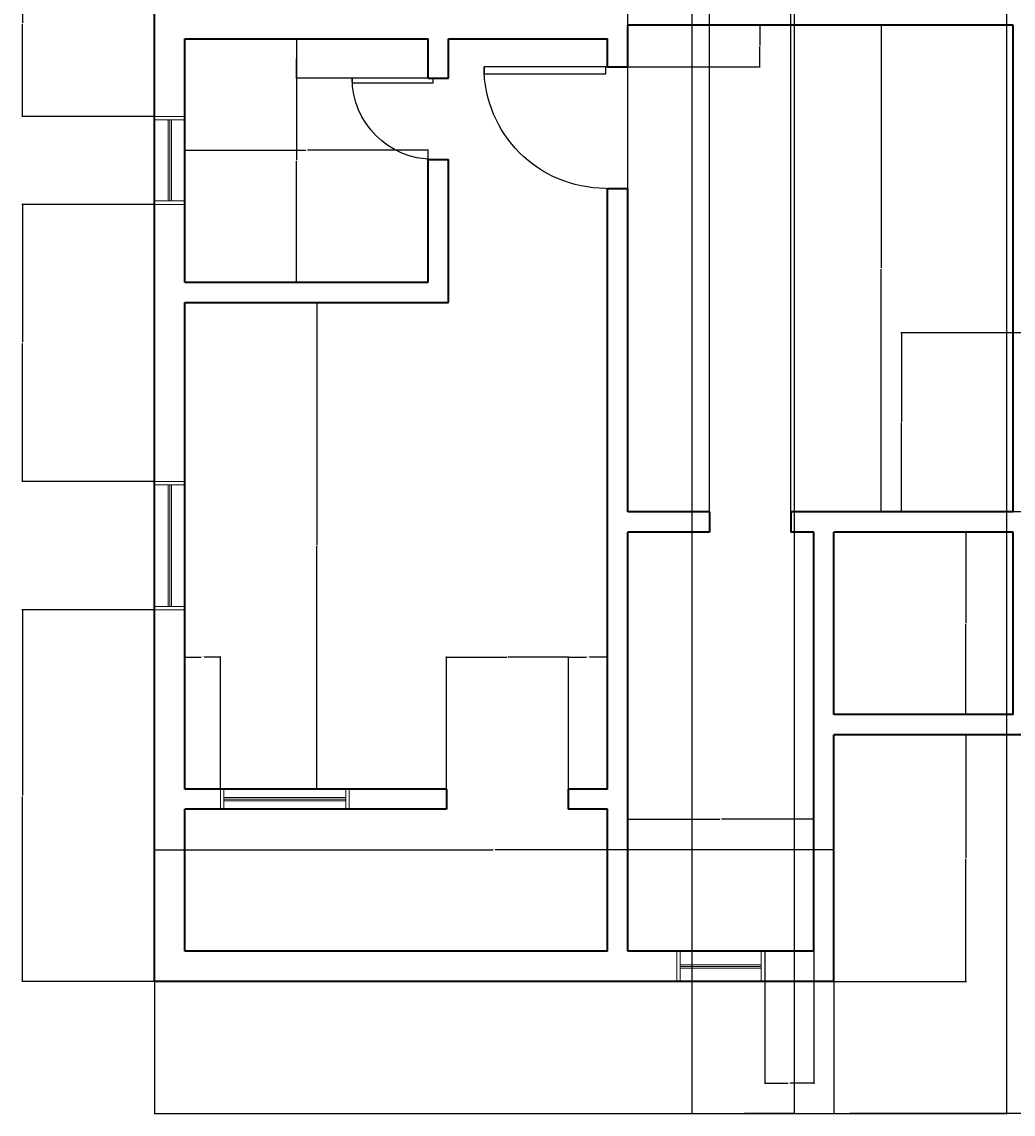
# Model space of a CAD drawing. Units: inches. Extents: x -7288 to -6705, y 7169 to 8028.
# Tile 1 of 5: x -7288 to -6995, y 7169 to 7493. Entities that reach past the tile are written whole.
import ezdxf

# ---------------------------------------------------------------- set-up
doc = ezdxf.new("R2010")
doc.units = ezdxf.units.IN
for name, color, linetype, lineweight in [('A-ANNO-DIMS', 2, 'Continuous', 18), ('A-DOOR', 3, 'Continuous', 25), ('A-GLAZ', 2, 'Continuous', 18), ('A-WALL', 1, 'Continuous', 35)]:
    doc.layers.add(name, color=color, linetype=linetype, lineweight=lineweight)
doc.styles.get("Standard").update_dxf_attribs({"font": 'arial.ttf'})
doc.dimstyles.get("Standard").update_dxf_attribs({"dimtxt": 0.18, "dimasz": 0.18, "dimexe": 0.18, "dimexo": 0.0625, "dimgap": 0.09, "dimtad": 0, "dimtih": 1, "dimtoh": 1, "dimdec": 4, "dimzin": 0, "dimdsep": 46, "dimtxsty": 'Standard', "dimcen": 0.09, "dimadec": 0, "dimazin": 0, "dimtfac": 1, "dimtdec": 4, "dimtofl": 0, "dimtmove": 0, "dimatfit": 3, "dimfxl": 1, "dimtolj": 1, "dimtzin": 0, "dimarcsym": 0})

# ---------------------------------------------------------------- blocks, each defined once
blk = doc.blocks.new('*U8')
for p, q in [((0, 0), (0, -100)), ((750, 0), (750, -100))]:
    blk.add_line(p, q)
blk.add_lwpolyline([(0, 0), (0, 750), (43.75, 750), (43.75, 0)], close=True)
blk.add_arc((0, 0), 750, 0, 90)
blk = doc.blocks.new('WIN-36IN-WALL9')
for p, q in [((0, 38), (9, 38)), ((0, 37), (9, 37)), ((4, 1), (4, 37)), ((4.5, 1), (4.5, 37)), ((5, 1), (5, 37)), ((0, 1), (9, 1)), ((0, 0), (9, 0))]:
    blk.add_line(p, q)
blk = doc.blocks.new('WIN-24IN-WALL9')
for p, q in [((0, 26), (9, 26)), ((0, 25), (9, 25)), ((4, 1), (4, 25)), ((4.5, 1), (4.5, 25)), ((5, 1), (5, 25)), ((0, 1), (9, 1)), ((0, 0), (9, 0))]:
    blk.add_line(p, q)
blk = doc.blocks.new('WIN-36IN-WALL6')
for p, q in [((0, 6), (0, 0)), ((1, 6), (1, 0)), ((1, 3.5), (37, 3.5)), ((37, 6), (37, 0)), ((38, 6), (38, 0)), ((1, 3), (37, 3)), ((1, 2.5), (37, 2.5))]:
    blk.add_line(p, q)
blk = doc.blocks.new('*D93')
at = {"layer": 'A-ANNO-DIMS', "color": 0, "lineweight": -2, "transparency": 16777216}
for p, q in [((-7248.84, 7208.47), (-7248.84, 7169.32)), ((-6744.84, 7208.47), (-6744.84, 7169.32)), ((-7248.66, 7169.5), (-6997.13, 7169.5)), ((-6745.02, 7169.5), (-6996.55, 7169.5))]:
    blk.add_line(p, q, dxfattribs=at)
at = {"layer": 'A-ANNO-DIMS', "color": 0, "transparency": 16777216}
for points in [[(-7248.66, 7169.53), (-7248.66, 7169.47), (-7248.84, 7169.5)], [(-6745.02, 7169.53), (-6745.02, 7169.47), (-6744.84, 7169.5)]]:
    blk.add_solid(points, dxfattribs=at)
at = {"layer": 'Defpoints', "color": 0, "transparency": 16777216}
for p in [(-7248.84, 7208.53), (-6744.84, 7208.53), (-6744.84, 7169.5)]:
    blk.add_point(p, dxfattribs=at)
at = {"layer": 'A-ANNO-DIMS', "color": 0, "transparency": 16777216, "insert": (-6996.84, 7169.5), "char_height": 0.18, "attachment_point": 5}
blk.add_mtext('\\A1;504', dxfattribs=at)
blk = doc.blocks.new('*D100')
at = {"layer": 'A-ANNO-DIMS', "color": 0, "lineweight": -2, "transparency": 16777216}
for p, q in [((-7248.84, 7208.59), (-7248.84, 7247.74)), ((-7248.66, 7247.56), (-7148.61, 7247.56)), ((-7048.02, 7247.56), (-7148.07, 7247.56)), ((-7047.84, 7208.59), (-7047.84, 7247.74))]:
    blk.add_line(p, q, dxfattribs=at)
at = {"layer": 'A-ANNO-DIMS', "color": 0, "transparency": 16777216}
for points in [[(-7248.66, 7247.59), (-7248.66, 7247.53), (-7248.84, 7247.56)], [(-7048.02, 7247.59), (-7048.02, 7247.53), (-7047.84, 7247.56)]]:
    blk.add_solid(points, dxfattribs=at)
at = {"layer": 'Defpoints', "color": 0, "transparency": 16777216}
for p in [(-7047.84, 7247.56), (-7248.84, 7208.53), (-7047.84, 7208.53)]:
    blk.add_point(p, dxfattribs=at)
at = {"layer": 'A-ANNO-DIMS', "color": 0, "transparency": 16777216, "insert": (-7148.34, 7247.56), "char_height": 0.18, "attachment_point": 5}
blk.add_mtext('\\A1;201', dxfattribs=at)
blk = doc.blocks.new('*D101')
at = {"layer": 'A-ANNO-DIMS', "color": 0, "lineweight": -2, "transparency": 16777216}
for p, q in [((-7047.84, 7208.47), (-7047.84, 7169.32)), ((-6945.84, 7208.47), (-6945.84, 7169.32)), ((-7047.66, 7169.5), (-6997.12, 7169.5)), ((-6946.02, 7169.5), (-6996.56, 7169.5))]:
    blk.add_line(p, q, dxfattribs=at)
at = {"layer": 'A-ANNO-DIMS', "color": 0, "transparency": 16777216}
for points in [[(-7047.66, 7169.53), (-7047.66, 7169.47), (-7047.84, 7169.5)], [(-6946.02, 7169.53), (-6946.02, 7169.47), (-6945.84, 7169.5)]]:
    blk.add_solid(points, dxfattribs=at)
at = {"layer": 'Defpoints', "color": 0, "transparency": 16777216}
for p in [(-7047.84, 7208.53), (-6945.84, 7208.53), (-6945.84, 7169.5)]:
    blk.add_point(p, dxfattribs=at)
at = {"layer": 'A-ANNO-DIMS', "color": 0, "transparency": 16777216, "insert": (-6996.84, 7169.5), "char_height": 0.18, "attachment_point": 5}
blk.add_mtext('\\A1;102', dxfattribs=at)
blk = doc.blocks.new('*D102')
at = {"layer": 'A-ANNO-DIMS', "color": 0, "lineweight": -2, "transparency": 16777216}
for p, q in [((-7047.78, 7281.53), (-7008.63, 7281.53)), ((-7008.81, 7281.35), (-7008.81, 7245.21)), ((-7008.81, 7208.71), (-7008.81, 7244.85)), ((-7047.78, 7208.53), (-7008.63, 7208.53))]:
    blk.add_line(p, q, dxfattribs=at)
at = {"layer": 'A-ANNO-DIMS', "color": 0, "transparency": 16777216}
for points in [[(-7008.84, 7281.35), (-7008.78, 7281.35), (-7008.81, 7281.53)], [(-7008.84, 7208.71), (-7008.78, 7208.71), (-7008.81, 7208.53)]]:
    blk.add_solid(points, dxfattribs=at)
at = {"layer": 'Defpoints', "color": 0, "transparency": 16777216}
for p in [(-7047.84, 7281.53), (-7047.84, 7208.53), (-7008.81, 7208.53)]:
    blk.add_point(p, dxfattribs=at)
at = {"layer": 'A-ANNO-DIMS', "color": 0, "transparency": 16777216, "insert": (-7008.81, 7245.03), "char_height": 0.18, "attachment_point": 5}
blk.add_mtext('\\A1;73', dxfattribs=at)
blk = doc.blocks.new('*D103')
at = {"layer": 'A-ANNO-DIMS', "color": 0, "lineweight": -2, "transparency": 16777216}
for p, q in [((-7089.84, 7838.47), (-7089.84, 7169.32)), ((-6996.84, 7838.47), (-6996.84, 7169.32)), ((-7089.66, 7169.5), (-7043.56, 7169.5)), ((-6997.02, 7169.5), (-7043.12, 7169.5))]:
    blk.add_line(p, q, dxfattribs=at)
at = {"layer": 'A-ANNO-DIMS', "color": 0, "transparency": 16777216}
for points in [[(-7089.66, 7169.53), (-7089.66, 7169.47), (-7089.84, 7169.5)], [(-6997.02, 7169.53), (-6997.02, 7169.47), (-6996.84, 7169.5)]]:
    blk.add_solid(points, dxfattribs=at)
at = {"layer": 'Defpoints', "color": 0, "transparency": 16777216}
for p in [(-7089.84, 7838.53), (-6996.84, 7838.53), (-6996.84, 7169.5)]:
    blk.add_point(p, dxfattribs=at)
at = {"layer": 'A-ANNO-DIMS', "color": 0, "transparency": 16777216, "insert": (-7043.34, 7169.5), "char_height": 0.18, "attachment_point": 5}
blk.add_mtext('\\A1;93', dxfattribs=at)
blk = doc.blocks.new('*D119')
at = {"layer": 'A-ANNO-DIMS', "color": 0, "lineweight": -2, "transparency": 16777216}
for p, q in [((-7089.84, 7799.47), (-7089.84, 7169.32)), ((-7059.61, 7799.47), (-7059.61, 7169.32)), ((-7089.66, 7169.5), (-7075.12, 7169.5)), ((-7059.79, 7169.5), (-7074.33, 7169.5))]:
    blk.add_line(p, q, dxfattribs=at)
at = {"layer": 'A-ANNO-DIMS', "color": 0, "transparency": 16777216}
for points in [[(-7089.66, 7169.53), (-7089.66, 7169.47), (-7089.84, 7169.5)], [(-7059.79, 7169.53), (-7059.79, 7169.47), (-7059.61, 7169.5)]]:
    blk.add_solid(points, dxfattribs=at)
at = {"layer": 'Defpoints', "color": 0, "transparency": 16777216}
for p in [(-7089.84, 7799.53), (-7059.61, 7799.53), (-7059.61, 7169.5)]:
    blk.add_point(p, dxfattribs=at)
at = {"layer": 'A-ANNO-DIMS', "color": 0, "transparency": 16777216, "insert": (-7074.72, 7169.5), "char_height": 0.18, "attachment_point": 5}
blk.add_mtext('\\A1;30.23', dxfattribs=at)
blk = doc.blocks.new('*D139')
at = {"layer": 'A-ANNO-DIMS', "color": 0, "lineweight": -2, "transparency": 16777216}
for p, q in [((-6994.9, 7491.53), (-7034.05, 7491.53)), ((-7033.87, 7491.35), (-7033.87, 7419.71)), ((-7033.87, 7347.71), (-7033.87, 7419.35)), ((-6994.9, 7347.53), (-7034.05, 7347.53))]:
    blk.add_line(p, q, dxfattribs=at)
at = {"layer": 'A-ANNO-DIMS', "color": 0, "transparency": 16777216}
for points in [[(-7033.9, 7491.35), (-7033.84, 7491.35), (-7033.87, 7491.53)], [(-7033.9, 7347.71), (-7033.84, 7347.71), (-7033.87, 7347.53)]]:
    blk.add_solid(points, dxfattribs=at)
at = {"layer": 'Defpoints', "color": 0, "transparency": 16777216}
for p in [(-7033.87, 7491.53), (-6994.84, 7491.53), (-6994.84, 7347.53)]:
    blk.add_point(p, dxfattribs=at)
at = {"layer": 'A-ANNO-DIMS', "color": 0, "transparency": 16777216, "insert": (-7033.87, 7419.53), "char_height": 0.18, "attachment_point": 5}
blk.add_mtext('\\A1;144', dxfattribs=at)
blk = doc.blocks.new('*D140')
at = {"layer": 'A-ANNO-DIMS', "color": 0, "lineweight": -2, "transparency": 16777216}
for p, q in [((-7239.84, 7415.59), (-7239.84, 7454.74)), ((-7239.66, 7454.56), (-7204.06, 7454.56)), ((-7168.02, 7454.56), (-7203.62, 7454.56)), ((-7167.84, 7415.59), (-7167.84, 7454.74))]:
    blk.add_line(p, q, dxfattribs=at)
at = {"layer": 'A-ANNO-DIMS', "color": 0, "transparency": 16777216}
for points in [[(-7239.66, 7454.59), (-7239.66, 7454.53), (-7239.84, 7454.56)], [(-7168.02, 7454.59), (-7168.02, 7454.53), (-7167.84, 7454.56)]]:
    blk.add_solid(points, dxfattribs=at)
at = {"layer": 'Defpoints', "color": 0, "transparency": 16777216}
for p in [(-7167.84, 7454.56), (-7239.84, 7415.53), (-7167.84, 7415.53)]:
    blk.add_point(p, dxfattribs=at)
at = {"layer": 'A-ANNO-DIMS', "color": 0, "transparency": 16777216, "insert": (-7203.84, 7454.56), "char_height": 0.18, "attachment_point": 5}
blk.add_mtext('\\A1;72', dxfattribs=at)
blk = doc.blocks.new('*D141')
at = {"layer": 'A-ANNO-DIMS', "color": 0, "lineweight": -2, "transparency": 16777216}
for p, q in [((-7167.9, 7487.53), (-7207.05, 7487.53)), ((-7206.87, 7487.35), (-7206.87, 7451.71)), ((-7206.87, 7415.71), (-7206.87, 7451.35)), ((-7167.9, 7415.53), (-7207.05, 7415.53))]:
    blk.add_line(p, q, dxfattribs=at)
at = {"layer": 'A-ANNO-DIMS', "color": 0, "transparency": 16777216}
for points in [[(-7206.9, 7487.35), (-7206.84, 7487.35), (-7206.87, 7487.53)], [(-7206.9, 7415.71), (-7206.84, 7415.71), (-7206.87, 7415.53)]]:
    blk.add_solid(points, dxfattribs=at)
at = {"layer": 'Defpoints', "color": 0, "transparency": 16777216}
for p in [(-7206.87, 7487.53), (-7167.84, 7487.53), (-7167.84, 7415.53)]:
    blk.add_point(p, dxfattribs=at)
at = {"layer": 'A-ANNO-DIMS', "color": 0, "transparency": 16777216, "insert": (-7206.87, 7451.53), "char_height": 0.18, "attachment_point": 5}
blk.add_mtext('\\A1;72', dxfattribs=at)
blk = doc.blocks.new('*D142')
at = {"layer": 'A-ANNO-DIMS', "color": 0, "lineweight": -2, "transparency": 16777216}
for p, q in [((-7239.78, 7409.53), (-7200.63, 7409.53)), ((-7200.81, 7409.35), (-7200.81, 7337.71)), ((-7200.81, 7265.71), (-7200.81, 7337.35)), ((-7239.78, 7265.53), (-7200.63, 7265.53))]:
    blk.add_line(p, q, dxfattribs=at)
at = {"layer": 'A-ANNO-DIMS', "color": 0, "transparency": 16777216}
for points in [[(-7200.84, 7409.35), (-7200.78, 7409.35), (-7200.81, 7409.53)], [(-7200.84, 7265.71), (-7200.78, 7265.71), (-7200.81, 7265.53)]]:
    blk.add_solid(points, dxfattribs=at)
at = {"layer": 'Defpoints', "color": 0, "transparency": 16777216}
for p in [(-7239.84, 7409.53), (-7239.84, 7265.53), (-7200.81, 7265.53)]:
    blk.add_point(p, dxfattribs=at)
at = {"layer": 'A-ANNO-DIMS', "color": 0, "transparency": 16777216, "insert": (-7200.81, 7337.53), "char_height": 0.18, "attachment_point": 5}
blk.add_mtext('\\A1;144', dxfattribs=at)
blk = doc.blocks.new('*D144')
at = {"layer": 'A-ANNO-DIMS', "color": 0, "lineweight": -2, "transparency": 16777216}
for p, q in [((-7108.84, 7217.59), (-7108.84, 7256.74)), ((-7108.66, 7256.56), (-7081.56, 7256.56)), ((-7054.02, 7256.56), (-7081.12, 7256.56)), ((-7053.84, 7217.59), (-7053.84, 7256.74))]:
    blk.add_line(p, q, dxfattribs=at)
at = {"layer": 'A-ANNO-DIMS', "color": 0, "transparency": 16777216}
for points in [[(-7108.66, 7256.59), (-7108.66, 7256.53), (-7108.84, 7256.56)], [(-7054.02, 7256.59), (-7054.02, 7256.53), (-7053.84, 7256.56)]]:
    blk.add_solid(points, dxfattribs=at)
at = {"layer": 'Defpoints', "color": 0, "transparency": 16777216}
for p in [(-7053.84, 7256.56), (-7108.84, 7217.53), (-7053.84, 7217.53)]:
    blk.add_point(p, dxfattribs=at)
at = {"layer": 'A-ANNO-DIMS', "color": 0, "transparency": 16777216, "insert": (-7081.34, 7256.56), "char_height": 0.18, "attachment_point": 5}
blk.add_mtext('\\A1;55', dxfattribs=at)
blk = doc.blocks.new('*D145')
at = {"layer": 'A-ANNO-DIMS', "color": 0, "lineweight": -2, "transparency": 16777216}
for p, q in [((-7047.78, 7341.53), (-7008.63, 7341.53)), ((-7008.81, 7341.35), (-7008.81, 7314.71)), ((-7008.81, 7287.71), (-7008.81, 7314.35)), ((-7047.78, 7287.53), (-7008.63, 7287.53))]:
    blk.add_line(p, q, dxfattribs=at)
at = {"layer": 'A-ANNO-DIMS', "color": 0, "transparency": 16777216}
for points in [[(-7008.84, 7341.35), (-7008.78, 7341.35), (-7008.81, 7341.53)], [(-7008.84, 7287.71), (-7008.78, 7287.71), (-7008.81, 7287.53)]]:
    blk.add_solid(points, dxfattribs=at)
at = {"layer": 'Defpoints', "color": 0, "transparency": 16777216}
for p in [(-7047.84, 7341.53), (-7047.84, 7287.53), (-7008.81, 7287.53)]:
    blk.add_point(p, dxfattribs=at)
at = {"layer": 'A-ANNO-DIMS', "color": 0, "transparency": 16777216, "insert": (-7008.81, 7314.53), "char_height": 0.18, "attachment_point": 5}
blk.add_mtext('\\A1;54', dxfattribs=at)
blk = doc.blocks.new('*D146')
at = {"layer": 'A-ANNO-DIMS', "color": 0, "lineweight": -2, "transparency": 16777216}
for p, q in [((-7248.9, 7318.53), (-7288.05, 7318.53)), ((-7287.87, 7318.35), (-7287.87, 7263.71)), ((-7287.87, 7208.71), (-7287.87, 7263.35)), ((-7248.9, 7208.53), (-7288.05, 7208.53))]:
    blk.add_line(p, q, dxfattribs=at)
at = {"layer": 'A-ANNO-DIMS', "color": 0, "transparency": 16777216}
for points in [[(-7287.9, 7318.35), (-7287.84, 7318.35), (-7287.87, 7318.53)], [(-7287.9, 7208.71), (-7287.84, 7208.71), (-7287.87, 7208.53)]]:
    blk.add_solid(points, dxfattribs=at)
at = {"layer": 'Defpoints', "color": 0, "transparency": 16777216}
for p in [(-7287.87, 7318.53), (-7248.84, 7318.53), (-7248.84, 7208.53)]:
    blk.add_point(p, dxfattribs=at)
at = {"layer": 'A-ANNO-DIMS', "color": 0, "transparency": 16777216, "insert": (-7287.87, 7263.53), "char_height": 0.18, "attachment_point": 5}
blk.add_mtext('\\A1;110', dxfattribs=at)
blk = doc.blocks.new('*D147')
at = {"layer": 'A-ANNO-DIMS', "color": 0, "lineweight": -2, "transparency": 16777216}
for p, q in [((-7248.9, 7438.53), (-7288.05, 7438.53)), ((-7287.87, 7438.35), (-7287.87, 7397.71)), ((-7287.87, 7356.71), (-7287.87, 7397.35)), ((-7248.9, 7356.53), (-7288.05, 7356.53))]:
    blk.add_line(p, q, dxfattribs=at)
at = {"layer": 'A-ANNO-DIMS', "color": 0, "transparency": 16777216}
for points in [[(-7287.9, 7438.35), (-7287.84, 7438.35), (-7287.87, 7438.53)], [(-7287.9, 7356.71), (-7287.84, 7356.71), (-7287.87, 7356.53)]]:
    blk.add_solid(points, dxfattribs=at)
at = {"layer": 'Defpoints', "color": 0, "transparency": 16777216}
for p in [(-7287.87, 7438.53), (-7248.84, 7438.53), (-7248.84, 7356.53)]:
    blk.add_point(p, dxfattribs=at)
at = {"layer": 'A-ANNO-DIMS', "color": 0, "transparency": 16777216, "insert": (-7287.87, 7397.53), "char_height": 0.18, "attachment_point": 5}
blk.add_mtext('\\A1;82', dxfattribs=at)
blk = doc.blocks.new('*D148')
at = {"layer": 'A-ANNO-DIMS', "color": 0, "lineweight": -2, "transparency": 16777216}
for p, q in [((-7248.9, 7519.53), (-7288.05, 7519.53)), ((-7287.87, 7519.35), (-7287.87, 7492.21)), ((-7287.87, 7464.71), (-7287.87, 7491.85)), ((-7248.9, 7464.53), (-7288.05, 7464.53))]:
    blk.add_line(p, q, dxfattribs=at)
at = {"layer": 'A-ANNO-DIMS', "color": 0, "transparency": 16777216}
for points in [[(-7287.9, 7519.35), (-7287.84, 7519.35), (-7287.87, 7519.53)], [(-7287.9, 7464.71), (-7287.84, 7464.71), (-7287.87, 7464.53)]]:
    blk.add_solid(points, dxfattribs=at)
at = {"layer": 'Defpoints', "color": 0, "transparency": 16777216}
for p in [(-7287.87, 7519.53), (-7248.84, 7519.53), (-7248.84, 7464.53)]:
    blk.add_point(p, dxfattribs=at)
at = {"layer": 'A-ANNO-DIMS', "color": 0, "transparency": 16777216, "insert": (-7287.87, 7492.03), "char_height": 0.18, "attachment_point": 5}
blk.add_mtext('\\A1;55', dxfattribs=at)
blk = doc.blocks.new('*D156')
at = {"layer": 'A-ANNO-DIMS', "color": 0, "lineweight": -2, "transparency": 16777216}
for p, q in [((-7084.64, 7347.59), (-7084.64, 8027.74)), ((-7084.46, 8027.56), (-7072.86, 8027.56)), ((-7060.82, 8027.56), (-7072.42, 8027.56)), ((-7060.64, 7347.59), (-7060.64, 8027.74))]:
    blk.add_line(p, q, dxfattribs=at)
at = {"layer": 'A-ANNO-DIMS', "color": 0, "transparency": 16777216}
for points in [[(-7084.46, 8027.59), (-7084.46, 8027.53), (-7084.64, 8027.56)], [(-7060.82, 8027.59), (-7060.82, 8027.53), (-7060.64, 8027.56)]]:
    blk.add_solid(points, dxfattribs=at)
at = {"layer": 'Defpoints', "color": 0, "transparency": 16777216}
for p in [(-7060.64, 8027.56), (-7084.64, 7347.53), (-7060.64, 7347.53)]:
    blk.add_point(p, dxfattribs=at)
at = {"layer": 'A-ANNO-DIMS', "color": 0, "transparency": 16777216, "insert": (-7072.64, 8027.56), "char_height": 0.18, "attachment_point": 5}
blk.add_mtext('\\A1;24', dxfattribs=at)
blk = doc.blocks.new('*D157')
at = {"layer": 'A-ANNO-DIMS', "color": 0, "lineweight": -2, "transparency": 16777216}
for p, q in [((-7108.84, 7347.59), (-7108.84, 8027.74)), ((-7108.66, 8027.56), (-7097.07, 8027.56)), ((-7084.82, 8027.56), (-7096.42, 8027.56)), ((-7084.64, 7347.59), (-7084.64, 8027.74))]:
    blk.add_line(p, q, dxfattribs=at)
at = {"layer": 'A-ANNO-DIMS', "color": 0, "transparency": 16777216}
for points in [[(-7108.66, 8027.59), (-7108.66, 8027.53), (-7108.84, 8027.56)], [(-7084.82, 8027.59), (-7084.82, 8027.53), (-7084.64, 8027.56)]]:
    blk.add_solid(points, dxfattribs=at)
at = {"layer": 'Defpoints', "color": 0, "transparency": 16777216}
for p in [(-7084.64, 8027.56), (-7108.84, 7347.53), (-7084.64, 7347.53)]:
    blk.add_point(p, dxfattribs=at)
at = {"layer": 'A-ANNO-DIMS', "color": 0, "transparency": 16777216, "insert": (-7096.74, 8027.56), "char_height": 0.18, "attachment_point": 5}
blk.add_mtext('\\A1;24.2', dxfattribs=at)
blk = doc.blocks.new('*D158')
at = {"layer": 'A-ANNO-DIMS', "color": 0, "lineweight": -2, "transparency": 16777216}
for p, q in [((-7068.34, 7217.47), (-7068.34, 7178.32)), ((-7053.84, 7217.47), (-7053.84, 7178.32)), ((-7068.16, 7178.5), (-7061.41, 7178.5)), ((-7054.02, 7178.5), (-7060.77, 7178.5))]:
    blk.add_line(p, q, dxfattribs=at)
at = {"layer": 'A-ANNO-DIMS', "color": 0, "transparency": 16777216}
for points in [[(-7068.16, 7178.53), (-7068.16, 7178.47), (-7068.34, 7178.5)], [(-7054.02, 7178.53), (-7054.02, 7178.47), (-7053.84, 7178.5)]]:
    blk.add_solid(points, dxfattribs=at)
at = {"layer": 'Defpoints', "color": 0, "transparency": 16777216}
for p in [(-7068.34, 7217.53), (-7053.84, 7217.53), (-7068.34, 7178.5)]:
    blk.add_point(p, dxfattribs=at)
at = {"layer": 'A-ANNO-DIMS', "color": 0, "transparency": 16777216, "insert": (-7061.09, 7178.5), "char_height": 0.18, "attachment_point": 5}
blk.add_mtext('\\A1;14.5', dxfattribs=at)
blk = doc.blocks.new('*D160')
at = {"layer": 'A-ANNO-DIMS', "color": 0, "lineweight": -2, "transparency": 16777216}
for p, q in [((-6988.9, 7400.53), (-7028.05, 7400.53)), ((-7027.87, 7400.35), (-7027.87, 7374.21)), ((-7027.87, 7347.71), (-7027.87, 7373.85)), ((-6988.9, 7347.53), (-7028.05, 7347.53))]:
    blk.add_line(p, q, dxfattribs=at)
at = {"layer": 'A-ANNO-DIMS', "color": 0, "transparency": 16777216}
for points in [[(-7027.9, 7400.35), (-7027.84, 7400.35), (-7027.87, 7400.53)], [(-7027.9, 7347.71), (-7027.84, 7347.71), (-7027.87, 7347.53)]]:
    blk.add_solid(points, dxfattribs=at)
at = {"layer": 'Defpoints', "color": 0, "transparency": 16777216}
for p in [(-7027.87, 7400.53), (-6988.84, 7400.53), (-6988.84, 7347.53)]:
    blk.add_point(p, dxfattribs=at)
at = {"layer": 'A-ANNO-DIMS', "color": 0, "transparency": 16777216, "insert": (-7027.87, 7374.03), "char_height": 0.18, "attachment_point": 5}
blk.add_mtext('\\A1;53', dxfattribs=at)
blk = doc.blocks.new('*D161')
at = {"layer": 'A-ANNO-DIMS', "color": 0, "lineweight": -2, "transparency": 16777216}
for p, q in [((-7239.84, 7265.59), (-7239.84, 7304.74)), ((-7239.66, 7304.56), (-7235.02, 7304.56)), ((-7229.46, 7304.56), (-7234.11, 7304.56)), ((-7229.28, 7265.59), (-7229.28, 7304.74))]:
    blk.add_line(p, q, dxfattribs=at)
at = {"layer": 'A-ANNO-DIMS', "color": 0, "transparency": 16777216}
for points in [[(-7239.66, 7304.59), (-7239.66, 7304.53), (-7239.84, 7304.56)], [(-7229.46, 7304.59), (-7229.46, 7304.53), (-7229.28, 7304.56)]]:
    blk.add_solid(points, dxfattribs=at)
at = {"layer": 'Defpoints', "color": 0, "transparency": 16777216}
for p in [(-7229.28, 7304.56), (-7239.84, 7265.53), (-7229.28, 7265.53)]:
    blk.add_point(p, dxfattribs=at)
at = {"layer": 'A-ANNO-DIMS', "color": 0, "transparency": 16777216, "insert": (-7234.56, 7304.56), "char_height": 0.18, "attachment_point": 5}
blk.add_mtext('\\A1;10.556', dxfattribs=at)
blk = doc.blocks.new('*D169')
at = {"layer": 'A-ANNO-DIMS', "color": 0, "lineweight": -2, "transparency": 16777216}
for p, q in [((-7108.78, 7491.53), (-7069.63, 7491.53)), ((-7069.81, 7491.35), (-7069.81, 7485.57)), ((-7069.81, 7479.43), (-7069.81, 7485.21)), ((-7108.78, 7479.25), (-7069.63, 7479.25))]:
    blk.add_line(p, q, dxfattribs=at)
at = {"layer": 'A-ANNO-DIMS', "color": 0, "transparency": 16777216}
for points in [[(-7069.84, 7491.35), (-7069.78, 7491.35), (-7069.81, 7491.53)], [(-7069.84, 7479.43), (-7069.78, 7479.43), (-7069.81, 7479.25)]]:
    blk.add_solid(points, dxfattribs=at)
at = {"layer": 'Defpoints', "color": 0, "transparency": 16777216}
for p in [(-7108.84, 7491.53), (-7108.84, 7479.25), (-7069.81, 7479.25)]:
    blk.add_point(p, dxfattribs=at)
at = {"layer": 'A-ANNO-DIMS', "color": 0, "transparency": 16777216, "insert": (-7069.81, 7485.39), "char_height": 0.18, "attachment_point": 5}
blk.add_mtext('\\A1;12.277', dxfattribs=at)
blk = doc.blocks.new('*D170')
at = {"layer": 'A-ANNO-DIMS', "color": 0, "lineweight": -2, "transparency": 16777216}
for p, q in [((-7167.9, 7487.53), (-7207.05, 7487.53)), ((-7206.87, 7487.35), (-7206.87, 7481.87)), ((-7206.87, 7476.02), (-7206.87, 7481.5)), ((-7167.9, 7475.84), (-7207.05, 7475.84))]:
    blk.add_line(p, q, dxfattribs=at)
at = {"layer": 'A-ANNO-DIMS', "color": 0, "transparency": 16777216}
for points in [[(-7206.9, 7487.35), (-7206.84, 7487.35), (-7206.87, 7487.53)], [(-7206.9, 7476.02), (-7206.84, 7476.02), (-7206.87, 7475.84)]]:
    blk.add_solid(points, dxfattribs=at)
at = {"layer": 'Defpoints', "color": 0, "transparency": 16777216}
for p in [(-7206.87, 7487.53), (-7167.84, 7487.53), (-7167.84, 7475.84)]:
    blk.add_point(p, dxfattribs=at)
at = {"layer": 'A-ANNO-DIMS', "color": 0, "transparency": 16777216, "insert": (-7206.87, 7481.68), "char_height": 0.18, "attachment_point": 5}
blk.add_mtext('\\A1;11.695', dxfattribs=at)
blk = doc.blocks.new('*D172')
at = {"layer": 'A-ANNO-DIMS', "color": 0, "lineweight": -2, "transparency": 16777216}
for p, q in [((-7162.42, 7265.59), (-7162.42, 7304.74)), ((-7162.24, 7304.56), (-7144.64, 7304.56)), ((-7126.6, 7304.56), (-7144.2, 7304.56)), ((-7126.42, 7265.59), (-7126.42, 7304.74))]:
    blk.add_line(p, q, dxfattribs=at)
at = {"layer": 'A-ANNO-DIMS', "color": 0, "transparency": 16777216}
for points in [[(-7162.24, 7304.59), (-7162.24, 7304.53), (-7162.42, 7304.56)], [(-7126.6, 7304.59), (-7126.6, 7304.53), (-7126.42, 7304.56)]]:
    blk.add_solid(points, dxfattribs=at)
at = {"layer": 'Defpoints', "color": 0, "transparency": 16777216}
for p in [(-7126.42, 7304.56), (-7162.42, 7265.53), (-7126.42, 7265.53)]:
    blk.add_point(p, dxfattribs=at)
at = {"layer": 'A-ANNO-DIMS', "color": 0, "transparency": 16777216, "insert": (-7144.42, 7304.56), "char_height": 0.18, "attachment_point": 5}
blk.add_mtext('\\A1;36', dxfattribs=at)
blk = doc.blocks.new('*D173')
at = {"layer": 'A-ANNO-DIMS', "color": 0, "lineweight": -2, "transparency": 16777216}
for p, q in [((-7126.42, 7265.59), (-7126.42, 7304.74)), ((-7126.24, 7304.56), (-7121.09, 7304.56)), ((-7115.02, 7304.56), (-7120.18, 7304.56)), ((-7114.84, 7265.59), (-7114.84, 7304.74))]:
    blk.add_line(p, q, dxfattribs=at)
at = {"layer": 'A-ANNO-DIMS', "color": 0, "transparency": 16777216}
for points in [[(-7126.24, 7304.59), (-7126.24, 7304.53), (-7126.42, 7304.56)], [(-7115.02, 7304.59), (-7115.02, 7304.53), (-7114.84, 7304.56)]]:
    blk.add_solid(points, dxfattribs=at)
at = {"layer": 'Defpoints', "color": 0, "transparency": 16777216}
for p in [(-7114.84, 7304.56), (-7126.42, 7265.53), (-7114.84, 7265.53)]:
    blk.add_point(p, dxfattribs=at)
at = {"layer": 'A-ANNO-DIMS', "color": 0, "transparency": 16777216, "insert": (-7120.63, 7304.56), "char_height": 0.18, "attachment_point": 5}
blk.add_mtext('\\A1;11.582', dxfattribs=at)

msp = doc.modelspace()

# ---------------------------------------------------------------- linework, layer by layer
at = {"layer": 'A-WALL'}
for p, q in [((-7248.8398, 7208.5311), (-7248.8398, 7958.5311)), ((-6994.8398, 7491.5311), (-7108.8398, 7491.5311)), ((-7108.8398, 7479.2542), (-7108.8398, 7491.5311)), ((-6994.8398, 7347.5311), (-6994.8398, 7491.5311)), ((-7239.8398, 7487.5311), (-7167.8398, 7487.5311)), ((-7239.8398, 7415.5311), (-7239.8398, 7487.5311)), ((-7167.8398, 7475.8361), (-7167.8398, 7487.5311)), ((-7161.8398, 7487.5311), (-7114.8398, 7487.5311)), ((-7161.8398, 7475.8361), (-7161.8398, 7487.5311)), ((-7114.8398, 7479.2542), (-7114.8398, 7487.5311)), ((-7114.8398, 7479.2542), (-7108.8398, 7479.2542)), ((-7167.8398, 7475.8361), (-7161.8398, 7475.8361)), ((-7167.8398, 7415.5311), (-7167.8398, 7451.8361)), ((-7167.8398, 7451.8361), (-7161.8398, 7451.8361)), ((-7161.8398, 7409.5311), (-7161.8398, 7451.8361)), ((-7114.8398, 7265.5311), (-7114.8398, 7443.2542)), ((-7114.8398, 7443.2542), (-7108.8398, 7443.2542)), ((-7108.8398, 7347.5311), (-7108.8398, 7443.2542)), ((-7239.8398, 7415.5311), (-7167.8398, 7415.5311)), ((-7239.8398, 7409.5311), (-7161.8398, 7409.5311)), ((-7239.8398, 7265.5311), (-7239.8398, 7409.5311)), ((-7084.6414, 7347.5311), (-7108.8398, 7347.5311)), ((-7084.6414, 7347.5311), (-7084.6414, 7341.5311)), ((-6994.8398, 7347.5311), (-7060.6414, 7347.5311)), ((-7060.6414, 7347.5311), (-7060.6414, 7341.5311)), ((-7108.8398, 7217.5311), (-7108.8398, 7341.5311)), ((-7084.6414, 7341.5311), (-7108.8398, 7341.5311)), ((-7053.8398, 7341.5311), (-7060.6414, 7341.5311)), ((-7053.8398, 7217.5311), (-7053.8398, 7341.5311)), ((-7047.8398, 7287.5311), (-7047.8398, 7341.5311)), ((-6994.8398, 7341.5311), (-7047.8398, 7341.5311)), ((-6994.8398, 7287.5311), (-6994.8398, 7341.5311)), ((-6994.8398, 7287.5311), (-7047.8398, 7287.5311)), ((-7047.8398, 7208.5311), (-7047.8398, 7281.5311)), ((-6945.8398, 7281.5311), (-7047.8398, 7281.5311)), ((-7162.4219, 7265.5311), (-7239.8398, 7265.5311)), ((-7162.4219, 7265.5311), (-7239.8398, 7265.5311)), ((-7162.4219, 7265.5311), (-7162.4219, 7259.5311)), ((-7114.8398, 7265.5311), (-7126.4219, 7265.5311)), ((-7114.8398, 7265.5311), (-7126.4219, 7265.5311)), ((-7126.4219, 7265.5311), (-7126.4219, 7259.5311)), ((-7239.8398, 7217.5311), (-7239.8398, 7259.5311)), ((-7162.4219, 7259.5311), (-7239.8398, 7259.5311)), ((-7162.4219, 7259.5311), (-7239.8398, 7259.5311)), ((-7114.8398, 7259.5311), (-7126.4219, 7259.5311)), ((-7114.8398, 7259.5311), (-7126.4219, 7259.5311)), ((-7114.8398, 7217.5311), (-7114.8398, 7259.5311)), ((-7114.8398, 7217.5311), (-7239.8398, 7217.5311)), ((-7053.8398, 7217.5311), (-7108.8398, 7217.5311)), ((-7047.8398, 7208.5311), (-7248.8398, 7208.5311))]:
    msp.add_line(p, q, dxfattribs=at)

# ---------------------------------------------------------------- block references
at = {"layer": 'A-DOOR', "rotation": 90}
for p, xscale, yscale, zscale in [((-7115.3659, 7479.252), -0.0479970023277597, 0.0479970023277597, 0.0479970023277597), ((-7166.3598, 7475.8361), -0.0320000000000005, 0.0320000000000005, 0.0320000000000005)]:
    msp.add_blockref('*U8', p, dxfattribs=dict(at, xscale=xscale, yscale=yscale, zscale=zscale))
at = {"layer": 'A-GLAZ'}
for name, p in [('WIN-24IN-WALL9', (-7248.8398, 7438.5311)), ('WIN-36IN-WALL6', (-7229.2839, 7259.5311))]:
    msp.add_blockref(name, p, dxfattribs=at)
for name, p, rotation in [('WIN-36IN-WALL9', (-7239.8398, 7356.5311), 180), ('WIN-24IN-WALL9', (-7094.3398, 7217.5311), 269.9999999999952)]:
    msp.add_blockref(name, p, dxfattribs=dict(at, rotation=rotation))

# ---------------------------------------------------------------- dimensions: what is measured, and where the dimension line sits
at = {"layer": 'A-ANNO-DIMS'}
for base, p1, p2, override, picture, middle in [((-7084.6414, 8027.5611), (-7108.8398, 7347.5311), (-7084.6414, 7347.5311), {"dimdec": 1, "dimlfac": 1, "dimrnd": 0, "dimzin": 0, "dimdsep": 46, "dimlunit": 2}, '*D157', (-7096.7406, 8027.5611)), ((-7060.6414, 8027.5611), (-7084.6414, 7347.5311), (-7060.6414, 7347.5311), {"dimdec": 0, "dimlfac": 1, "dimrnd": 0, "dimzin": 0, "dimdsep": 46, "dimlunit": 2}, '*D156', (-7072.6414, 8027.5611)), ((-6996.8398, 7169.5011), (-7089.8398, 7838.5311), (-6996.8398, 7838.5311), {"dimdec": 0, "dimlfac": 1, "dimrnd": 0, "dimzin": 0, "dimdsep": 46, "dimlunit": 2}, '*D103', (-7043.3398, 7169.5011)), ((-7059.607, 7169.5011), (-7089.8398, 7799.5311), (-7059.607, 7799.5311), {"dimdec": 2, "dimlfac": 1, "dimrnd": 0, "dimzin": 0, "dimdsep": 46, "dimlunit": 2}, '*D119', (-7074.7234, 7169.5011)), ((-7126.4219, 7304.5611), (-7162.4219, 7265.5311), (-7126.4219, 7265.5311), {"dimdec": 0, "dimlfac": 1, "dimrnd": 0, "dimzin": 0, "dimdsep": 46, "dimlunit": 2}, '*D172', (-7144.4219, 7304.5611)), ((-7114.8398, 7304.5611), (-7126.4219, 7265.5311), (-7114.8398, 7265.5311), {"dimdec": 3, "dimlfac": 1, "dimrnd": 0, "dimzin": 0, "dimdsep": 46, "dimlunit": 2}, '*D173', (-7120.6308, 7304.5611)), ((-7053.8398, 7256.5611), (-7108.8398, 7217.5311), (-7053.8398, 7217.5311), {"dimdec": 0, "dimlfac": 1, "dimrnd": 0, "dimzin": 0, "dimdsep": 46, "dimlunit": 2}, '*D144', (-7081.3398, 7256.5611)), ((-7047.8398, 7247.5611), (-7248.8398, 7208.5311), (-7047.8398, 7208.5311), {"dimdec": 0, "dimlfac": 1, "dimrnd": 0, "dimzin": 0, "dimdsep": 46, "dimlunit": 2}, '*D100', (-7148.3398, 7247.5611)), ((-6744.8398, 7169.5011), (-7248.8398, 7208.5311), (-6744.8398, 7208.5311), {"dimdec": 0, "dimlfac": 1, "dimrnd": 0, "dimzin": 0, "dimdsep": 46, "dimlunit": 2}, '*D93', (-6996.8398, 7169.5011)), ((-6945.8398, 7169.5011), (-7047.8398, 7208.5311), (-6945.8398, 7208.5311), {"dimdec": 0, "dimlfac": 1, "dimrnd": 0, "dimzin": 0, "dimdsep": 46, "dimlunit": 2}, '*D101', (-6996.8398, 7169.5011))]:
    dim = msp.add_linear_dim(base=base, p1=p1, p2=p2, dimstyle='Standard', override=override, dxfattribs=at)
    dim.commit()
    dim.dimension.update_dxf_attribs({"geometry": picture, "text_midpoint": middle})
for base, p1, p2, angle, override, picture, middle in [((-7287.8698, 7519.5311), (-7248.8398, 7464.5311), (-7248.8398, 7519.5311), 90, {"dimdec": 0, "dimlfac": 1, "dimrnd": 0, "dimzin": 0, "dimdsep": 46, "dimlunit": 2}, '*D148', (-7287.8698, 7492.0311)), ((-7069.8098, 7479.2542), (-7108.8398, 7491.5311), (-7108.8398, 7479.2542), 270, {"dimdec": 3, "dimlfac": 1, "dimrnd": 0, "dimzin": 0, "dimdsep": 46, "dimlunit": 2}, '*D169', (-7069.8098, 7485.3927)), ((-7033.8698, 7491.5311), (-6994.8398, 7347.5311), (-6994.8398, 7491.5311), 90, {"dimdec": 0, "dimlfac": 1, "dimrnd": 0, "dimzin": 0, "dimdsep": 46, "dimlunit": 2}, '*D139', (-7033.8698, 7419.5311)), ((-7206.8698, 7487.5311), (-7167.8398, 7475.8361), (-7167.8398, 7487.5311), 90, {"dimdec": 3, "dimlfac": 1, "dimrnd": 0, "dimzin": 0, "dimdsep": 46, "dimlunit": 2}, '*D170', (-7206.8698, 7481.6836)), ((-7206.8698, 7487.5311), (-7167.8398, 7415.5311), (-7167.8398, 7487.5311), 90, {"dimdec": 0, "dimlfac": 1, "dimrnd": 0, "dimzin": 0, "dimdsep": 46, "dimlunit": 2}, '*D141', (-7206.8698, 7451.5311)), ((-7167.8398, 7454.5611), (-7239.8398, 7415.5311), (-7167.8398, 7415.5311), 0, {"dimdec": 0, "dimlfac": 1, "dimrnd": 0, "dimzin": 0, "dimdsep": 46, "dimlunit": 2}, '*D140', (-7203.8398, 7454.5611)), ((-7287.8698, 7438.5311), (-7248.8398, 7356.5311), (-7248.8398, 7438.5311), 90, {"dimdec": 0, "dimlfac": 1, "dimrnd": 0, "dimzin": 0, "dimdsep": 46, "dimlunit": 2}, '*D147', (-7287.8698, 7397.5311)), ((-7200.8098, 7265.5311), (-7239.8398, 7409.5311), (-7239.8398, 7265.5311), 270, {"dimdec": 0, "dimlfac": 1, "dimrnd": 0, "dimzin": 0, "dimdsep": 46, "dimlunit": 2}, '*D142', (-7200.8098, 7337.5311)), ((-7027.8698, 7400.5311), (-6988.8398, 7347.5311), (-6988.8398, 7400.5311), 90, {"dimdec": 0, "dimlfac": 1, "dimrnd": 0, "dimzin": 0, "dimdsep": 46, "dimlunit": 2}, '*D160', (-7027.8698, 7374.0311)), ((-7008.8098, 7287.5311), (-7047.8398, 7341.5311), (-7047.8398, 7287.5311), 270, {"dimdec": 0, "dimlfac": 1, "dimrnd": 0, "dimzin": 0, "dimdsep": 46, "dimlunit": 2}, '*D145', (-7008.8098, 7314.5311)), ((-7287.8698, 7318.5311), (-7248.8398, 7208.5311), (-7248.8398, 7318.5311), 90, {"dimdec": 0, "dimlfac": 1, "dimrnd": 0, "dimzin": 0, "dimdsep": 46, "dimlunit": 2}, '*D146', (-7287.8698, 7263.5311)), ((-7229.2839, 7304.5611), (-7239.8398, 7265.5311), (-7229.2839, 7265.5311), 0, {"dimdec": 3, "dimlfac": 1, "dimrnd": 0, "dimzin": 0, "dimdsep": 46, "dimlunit": 2}, '*D161', (-7234.5619, 7304.5611)), ((-7008.8098, 7208.5311), (-7047.8398, 7281.5311), (-7047.8398, 7208.5311), 270, {"dimdec": 0, "dimlfac": 1, "dimrnd": 0, "dimzin": 0, "dimdsep": 46, "dimlunit": 2}, '*D102', (-7008.8098, 7245.0311)), ((-7068.3398, 7178.5011), (-7053.8398, 7217.5311), (-7068.3398, 7217.5311), 180, {"dimdec": 1, "dimlfac": 1, "dimrnd": 0, "dimzin": 0, "dimdsep": 46, "dimlunit": 2}, '*D158', (-7061.0898, 7178.5011))]:
    dim = msp.add_linear_dim(base=base, p1=p1, p2=p2, angle=angle, dimstyle='Standard', override=override, dxfattribs=at)
    dim.commit()
    dim.dimension.update_dxf_attribs({"geometry": picture, "text_midpoint": middle})

doc.saveas('drawing.dxf')
